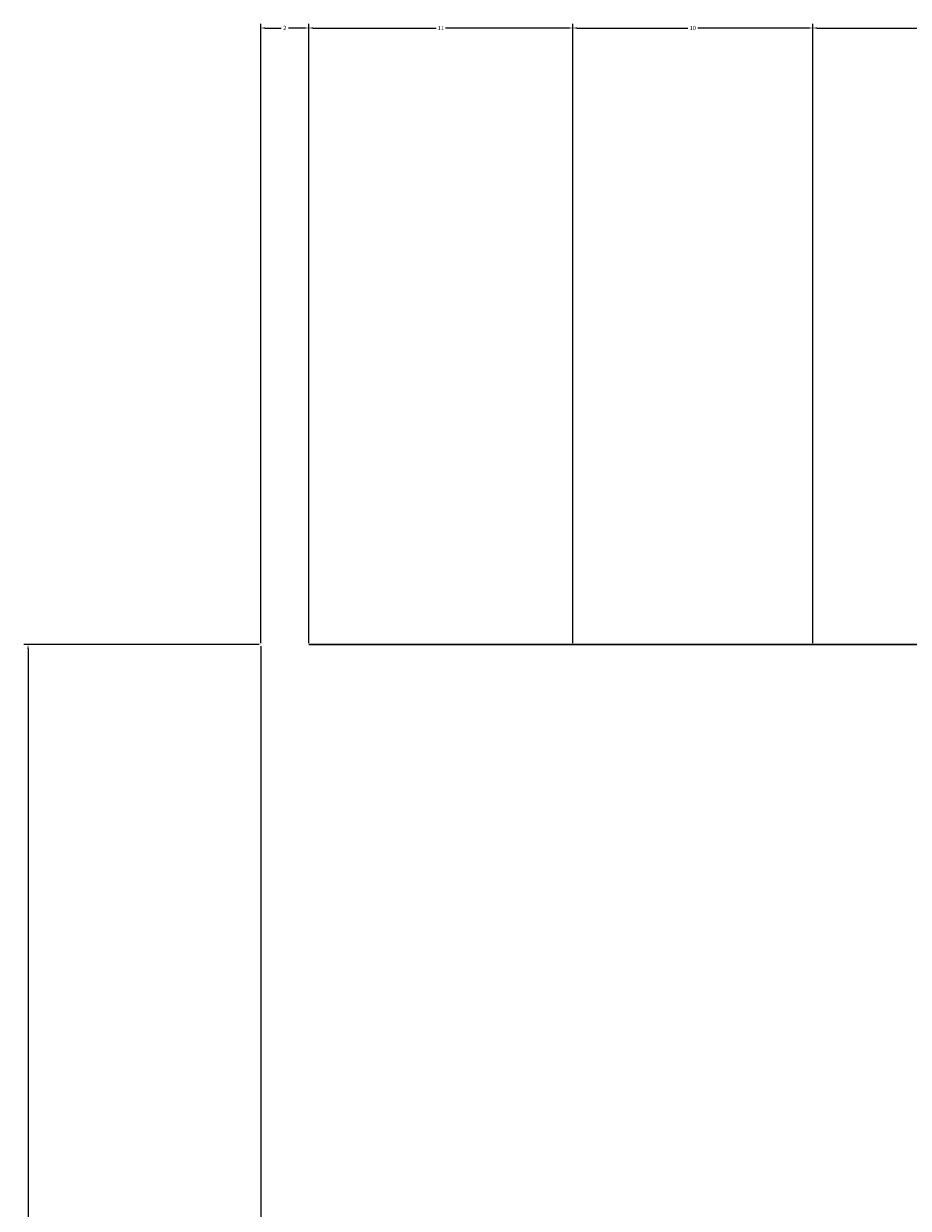
# Model space of a CAD drawing. Units: millimetres. Extents: x -136 to 10, y 158 to 257.
# Tile 2 of 6: x -136 to -99, y 208 to 257. Entities that reach past the tile are written whole.
import ezdxf

# ---------------------------------------------------------------- set-up
doc = ezdxf.new("R2010")
doc.units = ezdxf.units.MM
doc.layers.add('M-CONS', color=8, linetype='Continuous', lineweight=18)
doc.layers.add('M-DIMS', color=2, linetype='Continuous', lineweight=18)
doc.styles.get("Standard").update_dxf_attribs({"font": 'arial.ttf'})
doc.dimstyles.get("Standard").update_dxf_attribs({"dimtxt": 0.18, "dimasz": 0.18, "dimexe": 0.18, "dimexo": 0.0625, "dimgap": 0.09, "dimtad": 0, "dimtih": 1, "dimtoh": 1, "dimdec": 4, "dimzin": 0, "dimdsep": 46, "dimtxsty": 'Standard', "dimcen": 0.09, "dimadec": 0, "dimazin": 0, "dimtfac": 1, "dimtdec": 4, "dimtofl": 0, "dimtmove": 0, "dimatfit": 3, "dimfxl": 1, "dimtolj": 1, "dimtzin": 0, "dimarcsym": 0})

# ---------------------------------------------------------------- blocks, each defined once
blk = doc.blocks.new('*D1')
at = {"layer": 'Defpoints', "color": 0, "transparency": 16777216}
for p in [(-126, 231.107), (0, 231.107), (0, 158.407)]:
    blk.add_point(p, dxfattribs=at)
at = {"layer": 'M-DIMS', "color": 0, "lineweight": -2, "transparency": 16777216}
for p, q in [((-126, 231.044), (-126, 158.227)), ((0, 231.044), (0, 158.227)), ((-125.82, 158.407), (-63.28, 158.407)), ((-0.18, 158.407), (-62.72, 158.407))]:
    blk.add_line(p, q, dxfattribs=at)
at = {"layer": 'M-DIMS', "color": 0, "transparency": 16777216}
for points in [[(-125.82, 158.437), (-125.82, 158.377), (-126, 158.407)], [(-0.18, 158.437), (-0.18, 158.377), (0, 158.407)]]:
    blk.add_solid(points, dxfattribs=at)
at = {"layer": 'M-DIMS', "color": 0, "transparency": 16777216, "insert": (-63, 158.407), "char_height": 0.18, "attachment_point": 5}
blk.add_mtext('\\A1;126', dxfattribs=at)
blk = doc.blocks.new('*D3')
at = {"layer": 'Defpoints', "color": 0, "transparency": 16777216}
for p in [(-126, 231.107), (-135.7, 168.107), (-62.158, 168.107)]:
    blk.add_point(p, dxfattribs=at)
at = {"layer": 'M-DIMS', "color": 0, "lineweight": -2, "transparency": 16777216}
for p, q in [((-126.062, 231.107), (-135.88, 231.107)), ((-135.7, 230.927), (-135.7, 199.789)), ((-135.7, 168.287), (-135.7, 199.425)), ((-62.22, 168.107), (-135.88, 168.107))]:
    blk.add_line(p, q, dxfattribs=at)
at = {"layer": 'M-DIMS', "color": 0, "transparency": 16777216}
for points in [[(-135.73, 230.927), (-135.67, 230.927), (-135.7, 231.107)], [(-135.73, 168.287), (-135.67, 168.287), (-135.7, 168.107)]]:
    blk.add_solid(points, dxfattribs=at)
at = {"layer": 'M-DIMS', "color": 0, "transparency": 16777216, "insert": (-135.7, 199.607), "char_height": 0.18, "attachment_point": 5}
blk.add_mtext('\\A1;63', dxfattribs=at)
blk = doc.blocks.new('*D4')
at = {"layer": 'Defpoints', "color": 0, "transparency": 16777216}
for p in [(-124, 256.807), (-126, 231.107), (-124, 231.107)]:
    blk.add_point(p, dxfattribs=at)
at = {"layer": 'M-DIMS', "color": 0, "lineweight": -2, "transparency": 16777216}
for p, q in [((-126, 231.169), (-126, 256.987)), ((-125.82, 256.807), (-125.15, 256.807)), ((-124.18, 256.807), (-124.85, 256.807)), ((-124, 231.169), (-124, 256.987))]:
    blk.add_line(p, q, dxfattribs=at)
at = {"layer": 'M-DIMS', "color": 0, "transparency": 16777216}
for points in [[(-125.82, 256.837), (-125.82, 256.777), (-126, 256.807)], [(-124.18, 256.837), (-124.18, 256.777), (-124, 256.807)]]:
    blk.add_solid(points, dxfattribs=at)
at = {"layer": 'M-DIMS', "color": 0, "transparency": 16777216, "insert": (-125, 256.807), "char_height": 0.18, "attachment_point": 5}
blk.add_mtext('\\A1;2', dxfattribs=at)
blk = doc.blocks.new('*D5')
at = {"layer": 'Defpoints', "color": 0, "transparency": 16777216}
for p in [(-113, 256.807), (-124, 231.107), (-113, 231.107)]:
    blk.add_point(p, dxfattribs=at)
at = {"layer": 'M-DIMS', "color": 0, "lineweight": -2, "transparency": 16777216}
for p, q in [((-124, 231.169), (-124, 256.987)), ((-123.82, 256.807), (-118.693, 256.807)), ((-113.18, 256.807), (-118.307, 256.807)), ((-113, 231.169), (-113, 256.987))]:
    blk.add_line(p, q, dxfattribs=at)
at = {"layer": 'M-DIMS', "color": 0, "transparency": 16777216}
for points in [[(-123.82, 256.837), (-123.82, 256.777), (-124, 256.807)], [(-113.18, 256.837), (-113.18, 256.777), (-113, 256.807)]]:
    blk.add_solid(points, dxfattribs=at)
at = {"layer": 'M-DIMS', "color": 0, "transparency": 16777216, "insert": (-118.5, 256.807), "char_height": 0.18, "attachment_point": 5}
blk.add_mtext('\\A1;11', dxfattribs=at)
blk = doc.blocks.new('*D6')
at = {"layer": 'Defpoints', "color": 0, "transparency": 16777216}
for p in [(-103, 256.807), (-113, 231.107), (-103, 231.107)]:
    blk.add_point(p, dxfattribs=at)
at = {"layer": 'M-DIMS', "color": 0, "lineweight": -2, "transparency": 16777216}
for p, q in [((-113, 231.169), (-113, 256.987)), ((-112.82, 256.807), (-108.21, 256.807)), ((-103.18, 256.807), (-107.79, 256.807)), ((-103, 231.169), (-103, 256.987))]:
    blk.add_line(p, q, dxfattribs=at)
at = {"layer": 'M-DIMS', "color": 0, "transparency": 16777216}
for points in [[(-112.82, 256.837), (-112.82, 256.777), (-113, 256.807)], [(-103.18, 256.837), (-103.18, 256.777), (-103, 256.807)]]:
    blk.add_solid(points, dxfattribs=at)
at = {"layer": 'M-DIMS', "color": 0, "transparency": 16777216, "insert": (-108, 256.807), "char_height": 0.18, "attachment_point": 5}
blk.add_mtext('\\A1;10', dxfattribs=at)
blk = doc.blocks.new('*D7')
at = {"layer": 'Defpoints', "color": 0, "transparency": 16777216}
for p in [(-92, 256.807), (-103, 231.107), (-92, 231.107)]:
    blk.add_point(p, dxfattribs=at)
at = {"layer": 'M-DIMS', "color": 0, "lineweight": -2, "transparency": 16777216}
for p, q in [((-103, 231.169), (-103, 256.987)), ((-102.82, 256.807), (-97.693, 256.807)), ((-92.18, 256.807), (-97.307, 256.807)), ((-92, 231.169), (-92, 256.987))]:
    blk.add_line(p, q, dxfattribs=at)
at = {"layer": 'M-DIMS', "color": 0, "transparency": 16777216}
for points in [[(-102.82, 256.837), (-102.82, 256.777), (-103, 256.807)], [(-92.18, 256.837), (-92.18, 256.777), (-92, 256.807)]]:
    blk.add_solid(points, dxfattribs=at)
at = {"layer": 'M-DIMS', "color": 0, "transparency": 16777216, "insert": (-97.5, 256.807), "char_height": 0.18, "attachment_point": 5}
blk.add_mtext('\\A1;11', dxfattribs=at)

msp = doc.modelspace()

# ---------------------------------------------------------------- linework, layer by layer
at = {"layer": 'M-CONS', "extrusion": (0, -1, 0)}
msp.add_line((-126, 231.1068, 68.8035), (-126, 231.1068, 98.8035), dxfattribs=at)
for radius in [16, 5]:
    msp.add_circle((-108, 98.8035, -231.1068), radius, dxfattribs=at)

# ---------------------------------------------------------------- dimensions: what is measured, and where the dimension line sits
at = {"layer": 'M-DIMS'}
for base, p1, p2, picture, middle in [((-124, 256.8068), (-126, 231.1068), (-124, 231.1068), '*D4', (-125, 256.8068)), ((-113, 256.8068), (-124, 231.1068), (-113, 231.1068), '*D5', (-118.5, 256.8068)), ((-103, 256.8068), (-113, 231.1068), (-103, 231.1068), '*D6', (-108, 256.8068)), ((-92, 256.8068), (-103, 231.1068), (-92, 231.1068), '*D7', (-97.5, 256.8068)), ((0, 158.4068), (-126, 231.1068), (0, 231.1068), '*D1', (-63, 158.4068))]:
    dim = msp.add_linear_dim(base=base, p1=p1, p2=p2, dimstyle='Standard', override={"dimdec": 0, "dimlfac": 1, "dimrnd": 0, "dimzin": 0, "dimdsep": 46, "dimlunit": 2}, dxfattribs=at)
    dim.commit()
    dim.dimension.update_dxf_attribs({"geometry": picture, "text_midpoint": middle})
dim = msp.add_linear_dim(base=(-135.7, 168.1068), p1=(-126, 231.1068), p2=(-62.158, 168.1068), angle=90, dimstyle='Standard', override={"dimdec": 0, "dimlfac": 1, "dimrnd": 0, "dimzin": 0, "dimdsep": 46, "dimlunit": 2}, dxfattribs=at)
dim.commit()
dim.dimension.update_dxf_attribs({"geometry": '*D3', "text_midpoint": (-135.7, 199.6068)})

doc.saveas('drawing.dxf')
